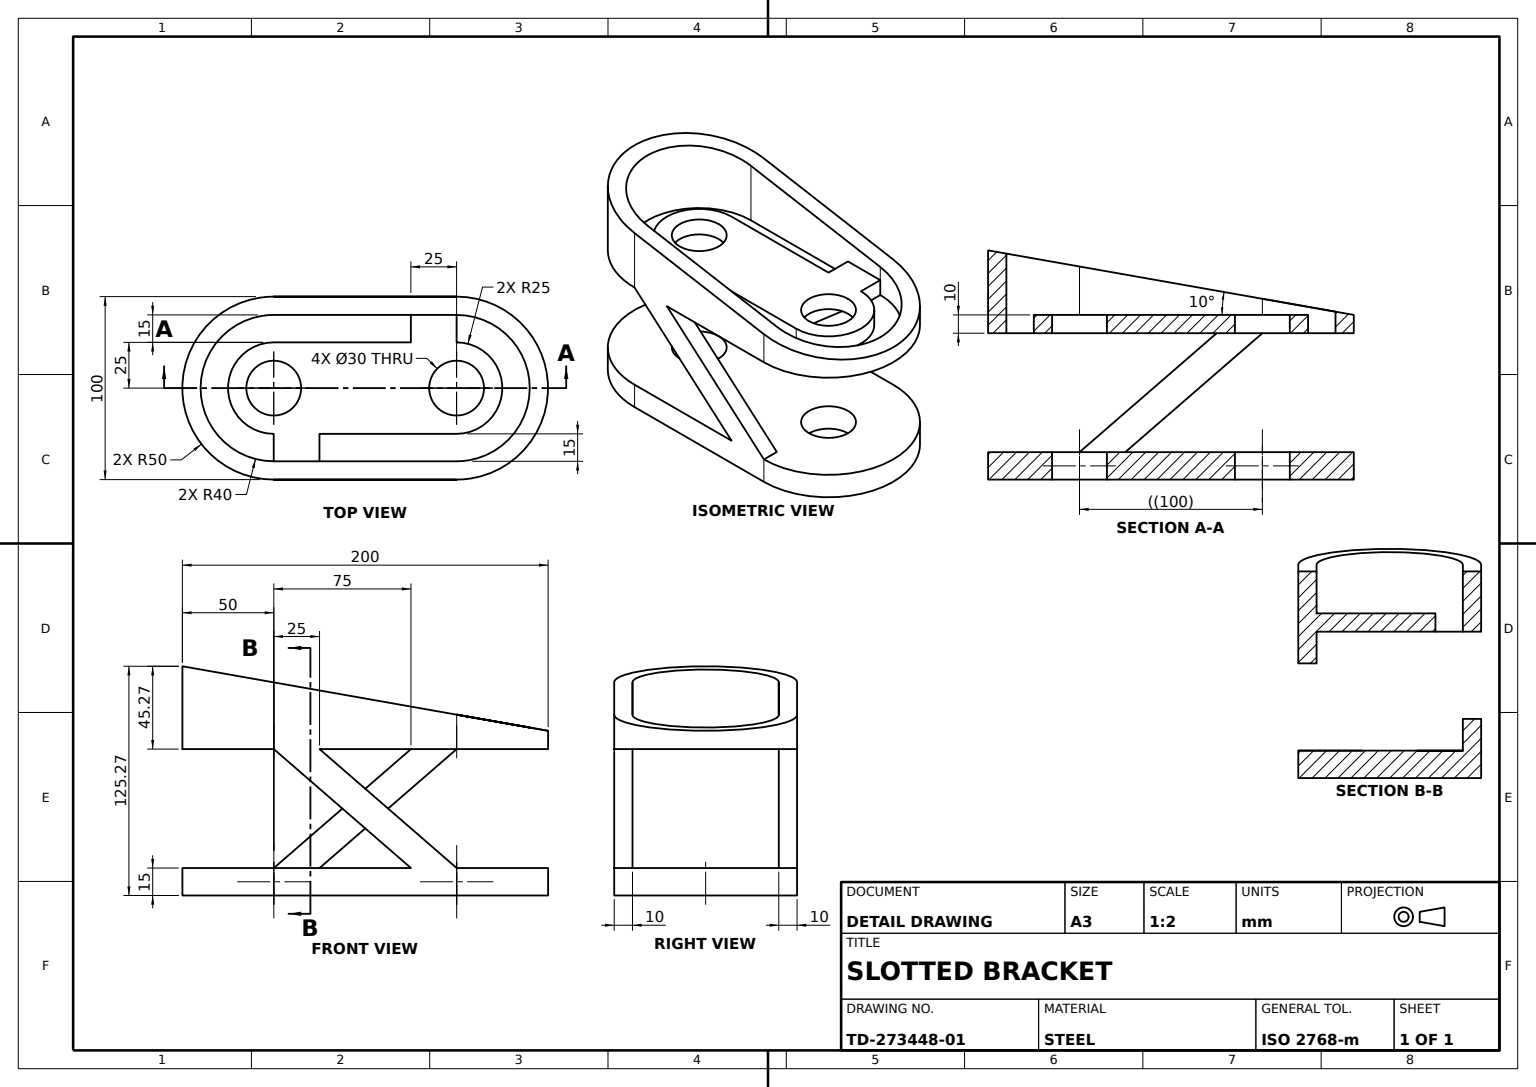
SolidWorks part; units mm, degrees
material "Plain Carbon Steel"
ref_plane "Front Plane" through (0, 0, 0) normal (0, 0, 1) x (1, 0, 0)
ref_plane "Top Plane" through (0, 0, 0) normal (0, 1, 0) x (1, 0, 0)
ref_plane "Right Plane" through (0, 0, 0) normal (1, 0, 0) x (0, 0, -1)
sketch "Base Plate Sketch" plane through (0, 0, 0) normal (0, 1, 0) x (1, 0, 0)
  line L0 (0, 0) -> (100, 0) construction
  line L1 (0, 50) -> (100, 50)
  line L2 (0, -50) -> (100, -50)
  arc A0 (0, 50) -> (0, -50) centre (0, 0) ccw
  arc A1 (100, -50) -> (100, 50) centre (100, 0) ccw
  point P3 (50, 0)
  dimension "D2" = 50
  dimension "D1" = 100
extrude "Base Plate" add sketch "Base Plate Sketch" along normal blind 15
sketch "Base Bore Sketch" plane through (0, 15, 0) normal (0, 1, 0) x (1, 0, 0)
  circle A0 centre (100, 0) radius 15
  circle A1 centre (0, 0) radius 15
  dimension "D1" = 30
extrude "Base Bore" cut sketch "Base Bore Sketch" against normal blind 15
ref_plane "Loop Plane 90mm" through (0, 90, 0) normal (0, 1, 0) x (1, 0, 0)
sketch "Loop Ring Sketch" plane through (0, 90, 0) normal (0, 1, 0) x (1, 0, 0)
  line L0 (0, -50) -> (100, -50) construction
  line L1 (100, 50) -> (0, 50) construction
  line L2 (0, -50) -> (100, -50)
  line L3 (100, 50) -> (0, 50)
  line L4 (0, 0) -> (100, 0) construction
  line L5 (0, 40) -> (100, 40)
  line L6 (0, -40) -> (100, -40)
  arc A0 (100, -50) -> (100, 50) centre (100, 0) ccw construction
  arc A1 (0, 50) -> (0, -50) centre (0, 0) ccw construction
  arc A2 (100, -50) -> (100, 50) centre (100, 0) ccw
  arc A3 (0, 50) -> (0, -50) centre (0, 0) ccw
  arc A4 (0, 40) -> (0, -40) centre (0, 0) ccw
  arc A5 (100, -40) -> (100, 40) centre (100, 0) ccw
  point P3 (50, 0)
  dimension "D1" = 40
extrude "Loop Ring" add sketch "Loop Ring Sketch" along normal blind 50 from offset 10 separate body offset against normal yes
sketch "Brace Angle Cut Sketch" plane through (0, 0, 50) normal (0, 0, 1) x (1, 0, 0)
  line L0 (150, 90) -> (150, 130)
  line L1 (150, 80) -> (150, 130) construction
  line L2 (150, 90) -> (-50, 125.2654)
  line L3 (0, 80) -> (100, 80) construction
  line L4 (150, 130) -> (100, 130) construction
  line L5 (150, 130) -> (-50, 130)
  line L6 (-50, 130) -> (-50, 125.2654)
  dimension "D1" = 10
  dimension "D2" = 10
  dimension "D3" = 4.7346
extrude "Brace Angle Cut" cut sketch "Brace Angle Cut Sketch" against normal through all
sketch "X-Brace Sketch" plane through (0, 90, 0) normal (0, 1, 0) x (1, 0, 0)
  line L0 (0, 0) -> (100, 0) construction
  line L1 (0, 25) -> (75, 25)
  line L2 (25, -25) -> (100, -25)
  line L3 (0, 40) -> (100, 40) construction
  line L5 (100, 25) -> (100, 40)
  line L6 (100, 40) -> (75, 40)
  line L7 (75, 25) -> (75, 40)
  line L8 (100, -40) -> (0, -40) construction
  line L10 (0, -25) -> (0, -40)
  line L11 (0, -40) -> (25, -40)
  line L12 (25, -25) -> (25, -40)
  arc A0 (0, 25) -> (0, -25) centre (0, 0) ccw
  arc A1 (100, -25) -> (100, 25) centre (100, 0) ccw
  point P4 (50, 0)
  dimension "D1" = 25
  dimension "D4" = 25
  dimension "D2" = 25
  dimension "D3" = 25
  dimension "D5" = 75
  dimension "D6" = 25
  dimension "D7" = 15
extrude "X-Brace Web" add sketch "X-Brace Sketch" against normal blind 10
sketch "Brace Trim Cut Sketch" plane through (0, 90, 0) normal (0, 1, 0) x (1, 0, 0)
  circle A0 centre (100, 0) radius 15 construction
  circle A1 centre (0, 0) radius 15 construction
  circle A2 centre (100, 0) radius 15
  circle A3 centre (0, 0) radius 15
extrude "Brace Trim Cut" cut sketch "Brace Trim Cut Sketch" against normal blind 10
sketch "Inner Plate Sketch" plane through (0, 0, 50) normal (0, 0, 1) x (1, 0, 0)
  line L0 (0, 80) -> (75, 15)
  line L1 (0, 15) -> (100, 15) construction
  line L2 (25, 80) -> (100, 15)
  line L3 (0, 80) -> (100, 80) construction
  line L4 (0, 80) -> (25, 80)
  line L5 (75, 15) -> (100, 15)
  dimension "D1" = 125
  dimension "D2" = 75
extrude "Inner Plate" add sketch "Inner Plate Sketch" against normal blind 10
sketch "Inner Plate Extension Sketch" plane through (0, 0, -50) normal (0, 0, -1) x (-1, 0, 0)
  line L0 (-100, 80) -> (-25, 15)
  line L1 (-100, 15) -> (0, 15) construction
  line L2 (-75, 80) -> (0, 15)
  line L3 (-100, 80) -> (0, 80) construction
  line L4 (-100, 80) -> (-75, 80)
  line L5 (-25, 15) -> (0, 15)
  dimension "D1" = 75
  dimension "D2" = 75
extrude "Inner Plate Extension" add sketch "Inner Plate Extension Sketch" against normal blind 10
